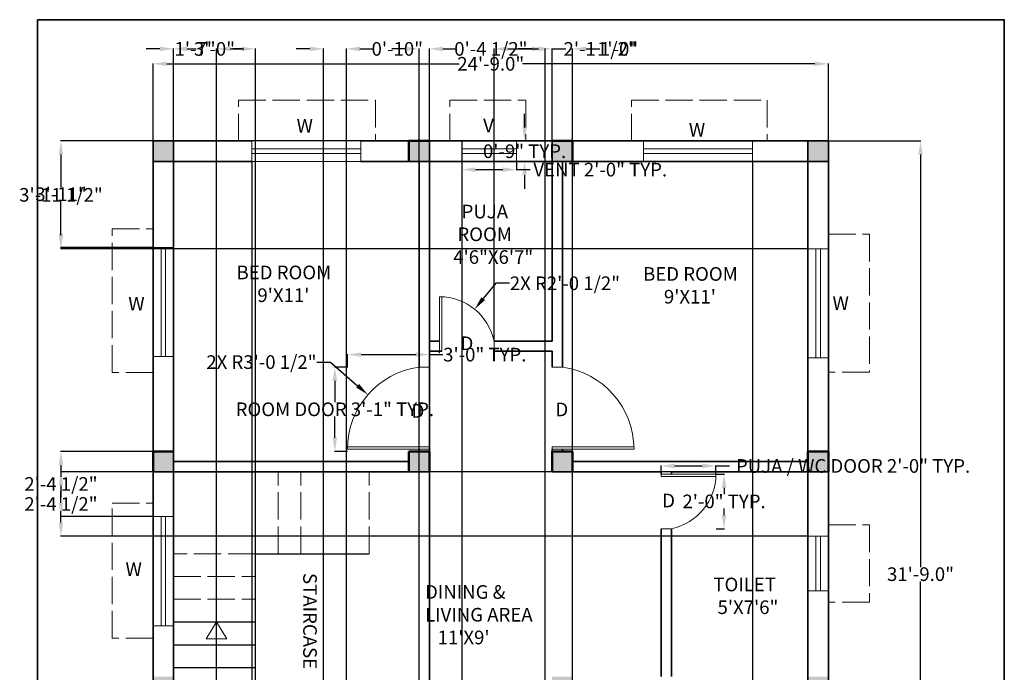
# Model space of a CAD drawing. Units: inches. Extents: x 730 to 1163, y 1530 to 2018.
# Tile 2 of 2: x 730 to 1163, y 1731 to 2018. Entities that reach past the tile are written whole.
import ezdxf

# ---------------------------------------------------------------- set-up
doc = ezdxf.new("R2010")
doc.units = ezdxf.units.IN
doc.header["$MEASUREMENT"] = 0
doc.linetypes.add('ACAD_ISO02W100', pattern=[15, 12, -3])
for name, color, linetype, lineweight in [('A-ANNO-DIMS', 2, 'Continuous', 18), ('A-ANNO-SYMB', 7, 'Continuous', 18), ('A-ANNO-TEXT', 7, 'Continuous', 18), ('A-ANNO-TTLB', 7, 'Continuous', 35), ('A-AREA-IDEN', 7, 'Continuous', 20), ('A-COLS', 7, 'Continuous', 50), ('A-COLS-PATT', 5, 'Continuous', 13), ('A-DOOR', 5, 'Continuous', 18), ('A-FLOR-STRS', 7, 'Continuous', 25), ('A-FLOR-STRS-OVHD', 7, 'ACAD_ISO02W100', 18), ('A-GLAZ', 5, 'Continuous', 18), ('A-GLAZ-OVHD', 7, 'ACAD_ISO02W100', 13), ('A-WALL', 7, 'Continuous', 35)]:
    doc.layers.add(name, color=color, linetype=linetype, lineweight=lineweight)
doc.styles.get("Standard").update_dxf_attribs({"font": 'arial.ttf'})
doc.dimstyles.get("Standard").update_dxf_attribs({"dimtxt": 6, "dimasz": 6, "dimexe": 0.18, "dimexo": 0.0625, "dimgap": 0.09, "dimtad": 0, "dimtih": 1, "dimtoh": 1, "dimdec": 1, "dimzin": 0, "dimdsep": 46, "dimlunit": 3, "dimtxsty": 'Standard', "dimcen": 0.09, "dimclrt": 1, "dimadec": 0, "dimazin": 0, "dimtfac": 1, "dimtdec": 1, "dimtofl": 0, "dimtmove": 0, "dimatfit": 3, "dimfxl": 1, "dimtolj": 1, "dimtzin": 0, "dimarcsym": 0})

# ---------------------------------------------------------------- blocks, each defined once
blk = doc.blocks.new('*D1')
at = {"layer": 'A-ANNO-DIMS', "color": 0, "lineweight": -2, "transparency": 16777216}
for p, q in [((788.44, 1964.64), (788.44, 1998.7)), ((794.44, 1998.52), (923, 1998.52)), ((1079.44, 1998.52), (950.88, 1998.52)), ((1085.44, 1964.64), (1085.44, 1998.7))]:
    blk.add_line(p, q, dxfattribs=at)
at = {"layer": 'A-ANNO-DIMS', "color": 0, "transparency": 16777216}
for points in [[(794.44, 1999.52), (794.44, 1997.52), (788.44, 1998.52)], [(1079.44, 1999.52), (1079.44, 1997.52), (1085.44, 1998.52)]]:
    blk.add_solid(points, dxfattribs=at)
at = {"layer": 'Defpoints', "color": 0, "transparency": 16777216}
for p in [(1085.44, 1998.52), (788.44, 1964.58), (1085.44, 1964.58)]:
    blk.add_point(p, dxfattribs=at)
at = {"layer": 'A-ANNO-DIMS', "color": 0, "transparency": 16777216, "insert": (936.94, 1998.52), "char_height": 6, "attachment_point": 5}
blk.add_mtext('\\A1;24\'-9.0"', dxfattribs=at)
blk = doc.blocks.new('*D2')
at = {"layer": 'A-ANNO-DIMS', "color": 0, "lineweight": -2, "transparency": 16777216}
for p, q in [((1085.5, 1964.58), (1126.1, 1964.58)), ((1125.92, 1958.58), (1125.92, 1777.23)), ((1125.92, 1589.58), (1125.92, 1770.92)), ((1085.5, 1583.58), (1126.1, 1583.58))]:
    blk.add_line(p, q, dxfattribs=at)
at = {"layer": 'A-ANNO-DIMS', "color": 0, "transparency": 16777216}
for points in [[(1124.92, 1958.58), (1126.92, 1958.58), (1125.92, 1964.58)], [(1124.92, 1589.58), (1126.92, 1589.58), (1125.92, 1583.58)]]:
    blk.add_solid(points, dxfattribs=at)
at = {"layer": 'Defpoints', "color": 0, "transparency": 16777216}
for p in [(1085.44, 1964.58), (1085.44, 1583.58), (1125.92, 1583.58)]:
    blk.add_point(p, dxfattribs=at)
at = {"layer": 'A-ANNO-DIMS', "color": 0, "transparency": 16777216, "insert": (1125.92, 1774.08), "char_height": 6, "attachment_point": 5}
blk.add_mtext('\\A1;31\'-9.0"', dxfattribs=at)
blk = doc.blocks.new('WINDOW-48IN')
for p, q in [((0, 9), (0, 0)), ((0, 9), (48, 9)), ((48, 0), (48, 9)), ((0, 5.5), (48, 5.5)), ((0, 3.5), (48, 3.5)), ((0, 0), (48, 0))]:
    blk.add_line(p, q)
blk = doc.blocks.new('VENT-24IN')
for p, q in [((0, 9), (0, 0)), ((24, 9), (0, 9)), ((24, 0), (24, 9)), ((24, 5.5), (0, 5.5)), ((0, 3.5), (24, 3.5)), ((0, 0), (24, 0))]:
    blk.add_line(p, q)
blk = doc.blocks.new('DOOR-SWING-36IN')
for p, q in [((36, 37), (31.5, 37)), ((0, 2), (36, 2)), ((36, 1), (0, 1)), ((0, 1), (36, 1)), ((36, 0), (36, 2))]:
    blk.add_line(p, q)
blk.add_arc((36.32, 1), 36.32, 97.6281, 180)
blk = doc.blocks.new('DOOR-SWING-24IN')
for p, q in [((0, 0), (0, 24)), ((0, 24), (0, 0)), ((1, 24), (1, 0)), ((24, 0), (24, 4.5))]:
    blk.add_line(p, q)
blk.add_arc((0, -0.52), 24.52, 11.8123, 90)
blk = doc.blocks.new('*D9')
at = {"layer": 'A-ANNO-DIMS', "color": 0, "lineweight": -2, "transparency": 16777216}
for p, q in [((924.22, 1955.51), (924.22, 1951.8)), ((948.22, 1955.51), (948.22, 1951.8)), ((930.22, 1951.98), (942.22, 1951.98)), ((948.22, 1951.98), (954.22, 1951.98))]:
    blk.add_line(p, q, dxfattribs=at)
at = {"layer": 'A-ANNO-DIMS', "color": 0, "transparency": 16777216}
for points in [[(930.22, 1952.98), (930.22, 1950.98), (924.22, 1951.98)], [(942.22, 1952.98), (942.22, 1950.98), (948.22, 1951.98)]]:
    blk.add_solid(points, dxfattribs=at)
at = {"layer": 'Defpoints', "color": 0, "transparency": 16777216}
for p in [(924.22, 1955.58), (948.22, 1955.58), (948.22, 1951.98)]:
    blk.add_point(p, dxfattribs=at)
at = {"layer": 'A-ANNO-DIMS', "color": 1, "transparency": 16777216, "insert": (985.09, 1951.98), "char_height": 6, "attachment_point": 5}
blk.add_mtext('\\A1;VENT 2\'-0" TYP.', dxfattribs=at)
blk = doc.blocks.new('*D10')
at = {"layer": 'A-ANNO-DIMS', "color": 0, "lineweight": -2, "transparency": 16777216}
for p, q in [((951.82, 1970.58), (951.82, 1976.58)), ((948.28, 1964.58), (952, 1964.58)), ((948.28, 1955.58), (952, 1955.58)), ((951.82, 1949.58), (951.82, 1943.58))]:
    blk.add_line(p, q, dxfattribs=at)
at = {"layer": 'A-ANNO-DIMS', "color": 0, "transparency": 16777216}
for points in [[(950.82, 1970.58), (952.82, 1970.58), (951.82, 1964.58)], [(950.82, 1949.58), (952.82, 1949.58), (951.82, 1955.58)]]:
    blk.add_solid(points, dxfattribs=at)
at = {"layer": 'Defpoints', "color": 0, "transparency": 16777216}
for p in [(948.22, 1964.58), (951.82, 1964.58), (948.22, 1955.58)]:
    blk.add_point(p, dxfattribs=at)
at = {"layer": 'A-ANNO-DIMS', "color": 1, "transparency": 16777216, "insert": (951.82, 1960.08), "char_height": 6, "attachment_point": 5}
blk.add_mtext('\\A1;0\'-9" TYP.', dxfattribs=at)
blk = doc.blocks.new('*D11')
at = {"layer": 'A-ANNO-DIMS', "color": 0, "lineweight": -2, "transparency": 16777216}
for p, q in [((873.88, 1865.08), (868.21, 1865.08)), ((868.39, 1859.08), (868.39, 1849.77)), ((868.39, 1834.08), (868.39, 1843.38)), ((873.88, 1828.08), (868.21, 1828.08))]:
    blk.add_line(p, q, dxfattribs=at)
at = {"layer": 'A-ANNO-DIMS', "color": 0, "transparency": 16777216}
for points in [[(867.39, 1859.08), (869.39, 1859.08), (868.39, 1865.08)], [(867.39, 1834.08), (869.39, 1834.08), (868.39, 1828.08)]]:
    blk.add_solid(points, dxfattribs=at)
at = {"layer": 'Defpoints', "color": 0, "transparency": 16777216}
for p in [(868.39, 1865.08), (873.94, 1865.08), (873.94, 1828.08)]:
    blk.add_point(p, dxfattribs=at)
at = {"layer": 'A-ANNO-DIMS', "color": 1, "transparency": 16777216, "insert": (868.39, 1846.58), "char_height": 6, "attachment_point": 5}
blk.add_mtext('\\A1;ROOM DOOR 3\'-1" TYP.', dxfattribs=at)
blk = doc.blocks.new('*D12')
at = {"layer": 'A-ANNO-DIMS', "color": 0, "lineweight": -2, "transparency": 16777216}
for p, q in [((873.94, 1865.14), (873.94, 1870.81)), ((879.94, 1870.63), (903.94, 1870.63)), ((909.94, 1865.14), (909.94, 1870.81)), ((909.94, 1870.63), (915.94, 1870.63))]:
    blk.add_line(p, q, dxfattribs=at)
at = {"layer": 'A-ANNO-DIMS', "color": 0, "transparency": 16777216}
for points in [[(879.94, 1871.63), (879.94, 1869.63), (873.94, 1870.63)], [(903.94, 1871.63), (903.94, 1869.63), (909.94, 1870.63)]]:
    blk.add_solid(points, dxfattribs=at)
at = {"layer": 'Defpoints', "color": 0, "transparency": 16777216}
for p in [(909.94, 1870.63), (873.94, 1865.08), (909.94, 1865.08)]:
    blk.add_point(p, dxfattribs=at)
at = {"layer": 'A-ANNO-DIMS', "color": 1, "transparency": 16777216, "insert": (934.32, 1870.63), "char_height": 6, "attachment_point": 5}
blk.add_mtext('\\A1;3\'-0" TYP.', dxfattribs=at)
blk = doc.blocks.new('*D13')
at = {"layer": 'A-ANNO-DIMS', "color": 0, "lineweight": -2, "transparency": 16777216}
for p, q in [((1011.94, 1818.14), (1011.94, 1821.86)), ((1017.94, 1821.68), (1029.94, 1821.68)), ((1035.94, 1818.14), (1035.94, 1821.86)), ((1035.94, 1821.68), (1041.94, 1821.68))]:
    blk.add_line(p, q, dxfattribs=at)
at = {"layer": 'A-ANNO-DIMS', "color": 0, "transparency": 16777216}
for points in [[(1017.94, 1822.68), (1017.94, 1820.68), (1011.94, 1821.68)], [(1029.94, 1822.68), (1029.94, 1820.68), (1035.94, 1821.68)]]:
    blk.add_solid(points, dxfattribs=at)
at = {"layer": 'Defpoints', "color": 0, "transparency": 16777216}
for p in [(1035.94, 1821.68), (1011.94, 1818.08), (1035.94, 1818.08)]:
    blk.add_point(p, dxfattribs=at)
at = {"layer": 'A-ANNO-DIMS', "color": 1, "transparency": 16777216, "insert": (1096.26, 1821.68), "char_height": 6, "attachment_point": 5}
blk.add_mtext('\\A1;PUJA / WC DOOR 2\'-0" TYP.', dxfattribs=at)
blk = doc.blocks.new('*D14')
at = {"layer": 'A-ANNO-DIMS', "color": 0, "lineweight": -2, "transparency": 16777216}
for p, q in [((1036, 1818.08), (1039.72, 1818.08)), ((1039.54, 1812.08), (1039.54, 1809.23)), ((1039.54, 1800.08), (1039.54, 1802.92)), ((1036, 1794.08), (1039.72, 1794.08))]:
    blk.add_line(p, q, dxfattribs=at)
at = {"layer": 'A-ANNO-DIMS', "color": 0, "transparency": 16777216}
for points in [[(1038.54, 1812.08), (1040.54, 1812.08), (1039.54, 1818.08)], [(1038.54, 1800.08), (1040.54, 1800.08), (1039.54, 1794.08)]]:
    blk.add_solid(points, dxfattribs=at)
at = {"layer": 'Defpoints', "color": 0, "transparency": 16777216}
for p in [(1035.94, 1818.08), (1035.94, 1794.08), (1039.54, 1794.08)]:
    blk.add_point(p, dxfattribs=at)
at = {"layer": 'A-ANNO-DIMS', "color": 1, "transparency": 16777216, "insert": (1039.54, 1806.08), "char_height": 6, "attachment_point": 5}
blk.add_mtext('\\A1;2\'-0" TYP.', dxfattribs=at)
blk = doc.blocks.new('*D15')
at = {"layer": 'A-ANNO-DIMS', "color": 0, "lineweight": -2, "transparency": 16777216}
for p, q in [((797.44, 1964.51), (797.44, 1540.9)), ((831.86, 1955.51), (831.86, 1540.9)), ((803.44, 1541.08), (825.86, 1541.08)), ((831.86, 1541.08), (837.86, 1541.08))]:
    blk.add_line(p, q, dxfattribs=at)
at = {"layer": 'A-ANNO-DIMS', "color": 0, "transparency": 16777216}
for points in [[(803.44, 1542.08), (803.44, 1540.08), (797.44, 1541.08)], [(825.86, 1542.08), (825.86, 1540.08), (831.86, 1541.08)]]:
    blk.add_solid(points, dxfattribs=at)
at = {"layer": 'Defpoints', "color": 0, "transparency": 16777216}
for p in [(797.44, 1964.58), (831.86, 1955.58), (831.86, 1541.08)]:
    blk.add_point(p, dxfattribs=at)
at = {"layer": 'A-ANNO-DIMS', "color": 1, "transparency": 16777216, "insert": (855.3, 1541.08), "char_height": 6, "attachment_point": 5}
blk.add_mtext('\\A1;2\'-10 1/2"', dxfattribs=at)
blk = doc.blocks.new('*D16')
at = {"layer": 'A-ANNO-DIMS', "color": 0, "lineweight": -2, "transparency": 16777216}
for p, q in [((909.94, 1964.51), (909.94, 1540.9)), ((924.22, 1964.51), (924.22, 1540.9)), ((915.94, 1541.08), (918.22, 1541.08)), ((924.22, 1541.08), (930.22, 1541.08))]:
    blk.add_line(p, q, dxfattribs=at)
at = {"layer": 'A-ANNO-DIMS', "color": 0, "transparency": 16777216}
for points in [[(915.94, 1542.08), (915.94, 1540.08), (909.94, 1541.08)], [(918.22, 1542.08), (918.22, 1540.08), (924.22, 1541.08)]]:
    blk.add_solid(points, dxfattribs=at)
at = {"layer": 'Defpoints', "color": 0, "transparency": 16777216}
for p in [(909.94, 1964.58), (924.22, 1964.58), (924.22, 1541.08)]:
    blk.add_point(p, dxfattribs=at)
at = {"layer": 'A-ANNO-DIMS', "color": 1, "transparency": 16777216, "insert": (944.99, 1541.08), "char_height": 6, "attachment_point": 5}
blk.add_mtext('\\A1;1\'-2 1/2"', dxfattribs=at)
blk = doc.blocks.new('*D17')
at = {"layer": 'A-ANNO-DIMS', "color": 0, "lineweight": -2, "transparency": 16777216}
for p, q in [((1076.44, 1964.51), (1076.44, 1540.9)), ((1052.04, 1955.51), (1052.04, 1540.9)), ((1058.04, 1541.08), (1070.44, 1541.08)), ((1076.44, 1541.08), (1082.44, 1541.08))]:
    blk.add_line(p, q, dxfattribs=at)
at = {"layer": 'A-ANNO-DIMS', "color": 0, "transparency": 16777216}
for points in [[(1058.04, 1542.08), (1058.04, 1540.08), (1052.04, 1541.08)], [(1070.44, 1542.08), (1070.44, 1540.08), (1076.44, 1541.08)]]:
    blk.add_solid(points, dxfattribs=at)
at = {"layer": 'Defpoints', "color": 0, "transparency": 16777216}
for p in [(1076.44, 1964.58), (1052.04, 1955.58), (1076.44, 1541.08)]:
    blk.add_point(p, dxfattribs=at)
at = {"layer": 'A-ANNO-DIMS', "color": 1, "transparency": 16777216, "insert": (1097.55, 1541.08), "char_height": 6, "attachment_point": 5}
blk.add_mtext('\\A1;2\'-0 1/2"', dxfattribs=at)
blk = doc.blocks.new('*D18')
at = {"layer": 'A-ANNO-DIMS', "color": 0, "lineweight": -2, "transparency": 16777216}
for p, q in [((788.38, 1964.58), (747.76, 1964.58)), ((747.94, 1958.58), (747.94, 1944.35)), ((747.94, 1923.81), (747.94, 1938.04)), ((788.38, 1917.81), (747.76, 1917.81))]:
    blk.add_line(p, q, dxfattribs=at)
at = {"layer": 'A-ANNO-DIMS', "color": 0, "transparency": 16777216}
for points in [[(746.94, 1958.58), (748.94, 1958.58), (747.94, 1964.58)], [(746.94, 1923.81), (748.94, 1923.81), (747.94, 1917.81)]]:
    blk.add_solid(points, dxfattribs=at)
at = {"layer": 'Defpoints', "color": 0, "transparency": 16777216}
for p in [(788.44, 1964.58), (747.94, 1917.81), (788.44, 1917.81)]:
    blk.add_point(p, dxfattribs=at)
at = {"layer": 'A-ANNO-DIMS', "color": 1, "transparency": 16777216, "insert": (747.94, 1941.19), "char_height": 6, "attachment_point": 5}
blk.add_mtext('\\A1;3\'-11"', dxfattribs=at)
blk = doc.blocks.new('*D19')
at = {"layer": 'A-ANNO-DIMS', "color": 0, "lineweight": -2, "transparency": 16777216}
for p, q in [((788.38, 1828.08), (747.76, 1828.08)), ((747.94, 1822.08), (747.94, 1816.93)), ((747.94, 1805.4), (747.94, 1810.54)), ((788.38, 1799.4), (747.76, 1799.4))]:
    blk.add_line(p, q, dxfattribs=at)
at = {"layer": 'A-ANNO-DIMS', "color": 0, "transparency": 16777216}
for points in [[(746.94, 1822.08), (748.94, 1822.08), (747.94, 1828.08)], [(746.94, 1805.4), (748.94, 1805.4), (747.94, 1799.4)]]:
    blk.add_solid(points, dxfattribs=at)
at = {"layer": 'Defpoints', "color": 0, "transparency": 16777216}
for p in [(788.44, 1828.08), (747.94, 1799.4), (788.44, 1799.4)]:
    blk.add_point(p, dxfattribs=at)
at = {"layer": 'A-ANNO-DIMS', "color": 1, "transparency": 16777216, "insert": (747.94, 1813.74), "char_height": 6, "attachment_point": 5}
blk.add_mtext('\\A1;2\'-4 1/2"', dxfattribs=at)
blk = doc.blocks.new('*D21')
at = {"layer": 'A-ANNO-DIMS', "color": 0, "lineweight": -2, "transparency": 16777216}
for p, q in [((1076.38, 1964.58), (747.76, 1964.58)), ((747.94, 1958.58), (747.94, 1944.08)), ((747.94, 1923.2), (747.94, 1937.69)), ((1076.38, 1917.2), (747.76, 1917.2))]:
    blk.add_line(p, q, dxfattribs=at)
at = {"layer": 'A-ANNO-DIMS', "color": 0, "transparency": 16777216}
for points in [[(746.94, 1958.58), (748.94, 1958.58), (747.94, 1964.58)], [(746.94, 1923.2), (748.94, 1923.2), (747.94, 1917.2)]]:
    blk.add_solid(points, dxfattribs=at)
at = {"layer": 'Defpoints', "color": 0, "transparency": 16777216}
for p in [(1076.44, 1964.58), (747.94, 1917.2), (1076.44, 1917.2)]:
    blk.add_point(p, dxfattribs=at)
at = {"layer": 'A-ANNO-DIMS', "color": 1, "transparency": 16777216, "insert": (747.94, 1940.89), "char_height": 6, "attachment_point": 5}
blk.add_mtext('\\A1;3\'-11 1/2"', dxfattribs=at)
blk = doc.blocks.new('*D22')
at = {"layer": 'A-ANNO-DIMS', "color": 0, "lineweight": -2, "transparency": 16777216}
for p, q in [((1076.38, 1819.08), (747.76, 1819.08)), ((747.94, 1813.08), (747.94, 1808.13)), ((747.94, 1796.8), (747.94, 1801.75)), ((1076.38, 1790.8), (747.76, 1790.8))]:
    blk.add_line(p, q, dxfattribs=at)
at = {"layer": 'A-ANNO-DIMS', "color": 0, "transparency": 16777216}
for points in [[(746.94, 1813.08), (748.94, 1813.08), (747.94, 1819.08)], [(746.94, 1796.8), (748.94, 1796.8), (747.94, 1790.8)]]:
    blk.add_solid(points, dxfattribs=at)
at = {"layer": 'Defpoints', "color": 0, "transparency": 16777216}
for p in [(747.94, 1819.08), (1076.44, 1819.08), (1076.44, 1790.8)]:
    blk.add_point(p, dxfattribs=at)
at = {"layer": 'A-ANNO-DIMS', "color": 1, "transparency": 16777216, "insert": (747.94, 1804.94), "char_height": 6, "attachment_point": 5}
blk.add_mtext('\\A1;2\'-4 1/2"', dxfattribs=at)
blk = doc.blocks.new('*D27')
at = {"layer": 'A-ANNO-DIMS', "color": 0, "lineweight": -2, "transparency": 16777216}
for p, q in [((797.44, 1733.14), (797.44, 2005.26)), ((803.44, 2005.08), (807.38, 2005.08)), ((827.44, 2005.08), (823.5, 2005.08)), ((833.44, 1733.14), (833.44, 2005.26))]:
    blk.add_line(p, q, dxfattribs=at)
at = {"layer": 'A-ANNO-DIMS', "color": 0, "transparency": 16777216}
for points in [[(803.44, 2006.08), (803.44, 2004.08), (797.44, 2005.08)], [(827.44, 2006.08), (827.44, 2004.08), (833.44, 2005.08)]]:
    blk.add_solid(points, dxfattribs=at)
at = {"layer": 'Defpoints', "color": 0, "transparency": 16777216}
for p in [(833.44, 2005.08), (797.44, 1733.08), (833.44, 1733.08)]:
    blk.add_point(p, dxfattribs=at)
at = {"layer": 'A-ANNO-DIMS', "color": 1, "transparency": 16777216, "insert": (815.44, 2005.08), "char_height": 6, "attachment_point": 5}
blk.add_mtext('\\A1;3\'-0"', dxfattribs=at)
blk = doc.blocks.new('*D28')
at = {"layer": 'A-ANNO-DIMS', "color": 0, "lineweight": -2, "transparency": 16777216}
for p, q in [((857.44, 2005.08), (851.44, 2005.08)), ((863.44, 1721.06), (863.44, 2005.26)), ((873.44, 1721.06), (873.44, 2005.26)), ((879.44, 2005.08), (885.44, 2005.08))]:
    blk.add_line(p, q, dxfattribs=at)
at = {"layer": 'A-ANNO-DIMS', "color": 0, "transparency": 16777216}
for points in [[(857.44, 2006.08), (857.44, 2004.08), (863.44, 2005.08)], [(879.44, 2006.08), (879.44, 2004.08), (873.44, 2005.08)]]:
    blk.add_solid(points, dxfattribs=at)
at = {"layer": 'Defpoints', "color": 0, "transparency": 16777216}
for p in [(873.44, 2005.08), (863.44, 1721), (873.44, 1721)]:
    blk.add_point(p, dxfattribs=at)
at = {"layer": 'A-ANNO-DIMS', "color": 1, "transparency": 16777216, "insert": (895.84, 2005.08), "char_height": 6, "attachment_point": 5}
blk.add_mtext('\\A1;0\'-10"', dxfattribs=at)
blk = doc.blocks.new('*D32')
at = {"layer": 'A-ANNO-DIMS', "color": 0, "lineweight": -2, "transparency": 16777216}
for p, q in [((791.44, 2005.08), (785.44, 2005.08)), ((797.44, 1605.26), (797.44, 2005.26)), ((816.4, 1613.85), (816.4, 2005.26)), ((822.4, 2005.08), (828.4, 2005.08))]:
    blk.add_line(p, q, dxfattribs=at)
at = {"layer": 'A-ANNO-DIMS', "color": 0, "transparency": 16777216}
for points in [[(791.44, 2006.08), (791.44, 2004.08), (797.44, 2005.08)], [(822.4, 2006.08), (822.4, 2004.08), (816.4, 2005.08)]]:
    blk.add_solid(points, dxfattribs=at)
at = {"layer": 'Defpoints', "color": 0, "transparency": 16777216}
for p in [(816.4, 2005.08), (816.4, 1613.79), (797.44, 1605.2)]:
    blk.add_point(p, dxfattribs=at)
at = {"layer": 'A-ANNO-DIMS', "color": 1, "transparency": 16777216, "insert": (806.92, 2005.08), "char_height": 6, "attachment_point": 5}
blk.add_mtext('\\A1;1\'-7"', dxfattribs=at)
blk = doc.blocks.new('*D34')
at = {"layer": 'A-ANNO-DIMS', "color": 0, "lineweight": -2, "transparency": 16777216}
for p, q in [((899.44, 2005.08), (893.44, 2005.08)), ((905.44, 1592.64), (905.44, 2005.26)), ((909.94, 1592.64), (909.94, 2005.26)), ((915.94, 2005.08), (921.94, 2005.08))]:
    blk.add_line(p, q, dxfattribs=at)
at = {"layer": 'A-ANNO-DIMS', "color": 0, "transparency": 16777216}
for points in [[(899.44, 2006.08), (899.44, 2004.08), (905.44, 2005.08)], [(915.94, 2006.08), (915.94, 2004.08), (909.94, 2005.08)]]:
    blk.add_solid(points, dxfattribs=at)
at = {"layer": 'Defpoints', "color": 0, "transparency": 16777216}
for p in [(909.94, 2005.08), (905.44, 1592.58), (909.94, 1592.58)]:
    blk.add_point(p, dxfattribs=at)
at = {"layer": 'A-ANNO-DIMS', "color": 1, "transparency": 16777216, "insert": (937, 2005.08), "char_height": 6, "attachment_point": 5}
blk.add_mtext('\\A1;0\'-4 1/2"', dxfattribs=at)
blk = doc.blocks.new('*D36')
at = {"layer": 'A-ANNO-DIMS', "color": 0, "lineweight": -2, "transparency": 16777216}
for p, q in [((954.94, 2005.08), (948.94, 2005.08)), ((960.94, 1583.64), (960.94, 2005.26)), ((972.94, 1583.64), (972.94, 2005.26)), ((978.94, 2005.08), (984.94, 2005.08))]:
    blk.add_line(p, q, dxfattribs=at)
at = {"layer": 'A-ANNO-DIMS', "color": 0, "transparency": 16777216}
for points in [[(954.94, 2006.08), (954.94, 2004.08), (960.94, 2005.08)], [(978.94, 2006.08), (978.94, 2004.08), (972.94, 2005.08)]]:
    blk.add_solid(points, dxfattribs=at)
at = {"layer": 'Defpoints', "color": 0, "transparency": 16777216}
for p in [(972.94, 2005.08), (960.94, 1583.58), (972.94, 1583.58)]:
    blk.add_point(p, dxfattribs=at)
at = {"layer": 'A-ANNO-DIMS', "color": 1, "transparency": 16777216, "insert": (992.72, 2005.08), "char_height": 6, "attachment_point": 5}
blk.add_mtext('\\A1;1\'-0"', dxfattribs=at)
blk = doc.blocks.new('*D37')
at = {"layer": 'A-ANNO-DIMS', "color": 0, "lineweight": -2, "transparency": 16777216}
for p, q in [((938.38, 1876.64), (938.38, 2005.26)), ((944.38, 2005.08), (957.94, 2005.08)), ((963.94, 1876.64), (963.94, 2005.26)), ((963.94, 2005.08), (969.94, 2005.08))]:
    blk.add_line(p, q, dxfattribs=at)
at = {"layer": 'A-ANNO-DIMS', "color": 0, "transparency": 16777216}
for points in [[(944.38, 2006.08), (944.38, 2004.08), (938.38, 2005.08)], [(957.94, 2006.08), (957.94, 2004.08), (963.94, 2005.08)]]:
    blk.add_solid(points, dxfattribs=at)
at = {"layer": 'Defpoints', "color": 0, "transparency": 16777216}
for p in [(963.94, 2005.08), (938.38, 1876.58), (963.94, 1876.58)]:
    blk.add_point(p, dxfattribs=at)
at = {"layer": 'A-ANNO-DIMS', "color": 1, "transparency": 16777216, "insert": (985.05, 2005.08), "char_height": 6, "attachment_point": 5}
blk.add_mtext('\\A1;2\'-1 1/2"', dxfattribs=at)
blk = doc.blocks.new('*D38')
at = {"layer": 'A-ANNO-DIMS', "color": 0, "lineweight": -2, "transparency": 16777216}
for p, q in [((860.53, 1867.35), (866.53, 1867.35)), ((866.53, 1867.35), (878.41, 1856.95)), ((910.17, 1829.08), (910.35, 1829.08)), ((910.26, 1828.99), (910.26, 1829.17))]:
    blk.add_line(p, q, dxfattribs=at)
at = {"layer": 'A-ANNO-DIMS', "color": 0, "transparency": 16777216}
blk.add_solid([(879.07, 1857.7), (877.76, 1856.19), (882.93, 1852.99)], dxfattribs=at)
at = {"layer": 'Defpoints', "color": 0, "transparency": 16777216}
for p in [(882.93, 1852.99), (910.26, 1829.08)]:
    blk.add_point(p, dxfattribs=at)
at = {"layer": 'A-ANNO-DIMS', "color": 1, "transparency": 16777216, "insert": (836.1, 1867.35), "char_height": 6, "attachment_point": 5}
blk.add_mtext('\\A1;2X R3\'-0 1/2"', dxfattribs=at)
blk = doc.blocks.new('*D40')
at = {"layer": 'A-ANNO-DIMS', "color": 0, "lineweight": -2, "transparency": 16777216}
for p, q in [((939.12, 1902.01), (933.63, 1895.24)), ((945.12, 1902.01), (939.12, 1902.01)), ((914.29, 1871.56), (914.47, 1871.56)), ((914.38, 1871.47), (914.38, 1871.65))]:
    blk.add_line(p, q, dxfattribs=at)
at = {"layer": 'A-ANNO-DIMS', "color": 0, "transparency": 16777216}
blk.add_solid([(932.85, 1895.87), (934.41, 1894.61), (929.85, 1890.59)], dxfattribs=at)
at = {"layer": 'Defpoints', "color": 0, "transparency": 16777216}
for p in [(929.85, 1890.59), (914.38, 1871.56)]:
    blk.add_point(p, dxfattribs=at)
at = {"layer": 'A-ANNO-DIMS', "color": 1, "transparency": 16777216, "insert": (969.55, 1902.01), "char_height": 6, "attachment_point": 5}
blk.add_mtext('\\A1;2X R2\'-0 1/2"', dxfattribs=at)

msp = doc.modelspace()

# ---------------------------------------------------------------- hatches: boundary and pattern name
at = {"layer": 'A-COLS-PATT'}
h = msp.add_hatch(color=256, dxfattribs=at)
h.dxf.hatch_style = 1
h.paths.add_polyline_path([(797.44, 1964.58), (788.44, 1964.58), (788.44, 1955.58), (797.44, 1955.58)])
h.paths.add_polyline_path([(909.94, 1964.58), (900.94, 1964.58), (900.94, 1955.58), (909.94, 1955.58)])
h.paths.add_polyline_path([(972.94, 1964.58), (963.94, 1964.58), (963.94, 1955.58), (972.94, 1955.58)])
h.paths.add_polyline_path([(1085.44, 1964.58), (1076.44, 1964.58), (1076.44, 1955.58), (1085.44, 1955.58)])
h.paths.add_polyline_path([(797.44, 1828.08), (788.44, 1828.08), (788.44, 1819.08), (797.44, 1819.08)])
h.paths.add_polyline_path([(909.94, 1828.08), (900.94, 1828.08), (900.94, 1819.08), (909.94, 1819.08)])
h.paths.add_polyline_path([(972.94, 1828.08), (963.94, 1828.08), (963.94, 1819.08), (972.94, 1819.08)])
h.paths.add_polyline_path([(1085.44, 1828.08), (1076.44, 1828.08), (1076.44, 1819.08), (1085.44, 1819.08)])
h.paths.add_polyline_path([(797.44, 1729.08), (788.44, 1729.08), (788.44, 1720.08), (797.44, 1720.08)])
h.paths.add_polyline_path([(972.96, 1729.08), (963.94, 1729.08), (963.94, 1720.07), (972.96, 1720.07)])
h.paths.add_polyline_path([(1085.44, 1729.08), (1076.44, 1729.08), (1076.44, 1720.08), (1085.44, 1720.08)])
h.paths.add_polyline_path([(1085.44, 1592.58), (1076.44, 1592.58), (1076.44, 1583.58), (1085.44, 1583.58)])
h.paths.add_polyline_path([(972.94, 1592.58), (963.94, 1592.58), (963.94, 1583.58), (972.94, 1583.58)])
h.paths.add_polyline_path([(909.94, 1592.58), (900.94, 1592.58), (900.94, 1583.58), (909.94, 1583.58)])
h.paths.add_polyline_path([(797.44, 1592.58), (788.44, 1592.58), (788.44, 1583.58), (797.44, 1583.58)])

# ---------------------------------------------------------------- linework, layer by layer
at = {"layer": 'A-ANNO-SYMB'}
for p, q in [((816.36, 1753.08), (811.77, 1745.67)), ((816.36, 1753.08), (820.95, 1745.67)), ((811.77, 1745.67), (820.95, 1745.67)), ((816.36, 1701.04), (816.36, 1745.67))]:
    msp.add_line(p, q, dxfattribs=at)
at = {"layer": 'A-ANNO-TTLB'}
msp.add_lwpolyline([(737.62, 2017.92), (1162.77, 2017.92), (1162.77, 1530.25), (737.62, 1530.25)], close=True, dxfattribs=at)
at = {"layer": 'A-COLS'}
for p, q in [((909.94, 1964.58), (900.94, 1964.58)), ((900.94, 1964.58), (900.94, 1955.58)), ((963.94, 1964.58), (972.94, 1964.58)), ((972.94, 1964.58), (972.94, 1955.58)), ((788.44, 1819.08), (788.44, 1828.08)), ((788.44, 1828.08), (797.44, 1828.08)), ((909.94, 1828.08), (900.94, 1828.08)), ((900.94, 1828.08), (900.94, 1819.08)), ((909.94, 1819.08), (909.94, 1828.08)), ((963.94, 1819.08), (963.94, 1828.08)), ((963.94, 1828.08), (972.94, 1828.08)), ((972.94, 1828.08), (972.94, 1819.08)), ((1085.44, 1828.08), (1076.44, 1828.08)), ((1076.44, 1828.08), (1076.44, 1819.08)), ((1085.44, 1819.08), (1085.44, 1828.08))]:
    msp.add_line(p, q, dxfattribs=at)
at = {"layer": 'A-DOOR'}
msp.add_line((1011.94, 1819.08), (1011.94, 1817.08), dxfattribs=at)
at = {"layer": 'A-FLOR-STRS'}
for p, q in [((797.44, 1819.08), (797.44, 1783.08)), ((833.44, 1783.08), (883.44, 1783.08)), ((833.44, 1681.08), (833.44, 1783.08)), ((797.44, 1753.08), (833.44, 1753.08)), ((797.44, 1743.08), (833.44, 1743.08)), ((797.44, 1733.08), (833.44, 1733.08))]:
    msp.add_line(p, q, dxfattribs=at)
at = {"layer": 'A-FLOR-STRS-OVHD'}
for p, q in [((833.44, 1783.08), (833.44, 1819.08)), ((843.44, 1783.08), (843.44, 1819.08)), ((853.44, 1783.08), (853.44, 1819.08)), ((863.44, 1783.08), (863.44, 1819.08)), ((873.44, 1783.08), (873.44, 1819.08)), ((883.44, 1783.08), (883.44, 1819.08)), ((833.44, 1783.08), (797.44, 1783.08)), ((797.44, 1773.08), (833.44, 1773.08)), ((797.44, 1763.08), (833.44, 1763.08))]:
    msp.add_line(p, q, dxfattribs=at)
at = {"layer": 'A-GLAZ-OVHD'}
for p, q in [((826.03, 1964.58), (826.03, 1982.58)), ((826.03, 1982.58), (886.23, 1982.58)), ((886.23, 1982.58), (886.23, 1964.58)), ((918.9, 1964.58), (918.9, 1982.58)), ((918.9, 1982.58), (952.44, 1982.58)), ((952.44, 1982.58), (952.44, 1964.58)), ((998.8, 1964.58), (998.8, 1982.58)), ((998.8, 1982.58), (1058.55, 1982.58)), ((1058.55, 1982.58), (1058.55, 1964.58)), ((770.44, 1862.84), (770.44, 1925.89)), ((770.44, 1925.89), (788.44, 1925.89)), ((1085.44, 1923.62), (1103.44, 1923.62)), ((1103.44, 1923.62), (1103.44, 1862.96)), ((788.44, 1862.84), (770.44, 1862.84)), ((1103.44, 1862.96), (1085.44, 1862.96)), ((770.44, 1745.93), (770.44, 1805.25)), ((770.44, 1805.25), (788.44, 1805.25)), ((1085.44, 1795.74), (1103.44, 1795.74)), ((1103.44, 1795.74), (1103.44, 1761.8)), ((1103.44, 1761.8), (1085.44, 1761.8)), ((788.44, 1745.93), (770.44, 1745.93))]:
    msp.add_line(p, q, dxfattribs=at)
at = {"layer": 'A-WALL'}
for p, q in [((788.44, 1964.58), (831.86, 1964.58)), ((788.44, 1964.58), (788.44, 1583.58)), ((797.44, 1964.58), (797.44, 1681.08)), ((879.86, 1964.58), (1085.44, 1964.58)), ((909.94, 1964.58), (909.94, 1876.58)), ((963.94, 1964.58), (963.94, 1876.58)), ((1076.44, 1964.58), (1076.44, 1583.58)), ((1085.44, 1964.58), (1085.44, 1583.58)), ((788.44, 1955.58), (831.86, 1955.58)), ((879.86, 1955.58), (1085.44, 1955.58)), ((905.44, 1955.58), (905.44, 1865.08)), ((968.44, 1955.58), (968.44, 1865.08)), ((909.94, 1876.58), (914.38, 1876.58)), ((938.38, 1876.58), (963.94, 1876.58)), ((909.94, 1872.08), (915.38, 1872.08)), ((909.94, 1872.08), (909.94, 1865.08)), ((938.38, 1872.08), (963.94, 1872.08)), ((963.94, 1872.08), (963.94, 1865.08)), ((905.44, 1829.08), (905.44, 1828.08)), ((909.94, 1829.08), (909.94, 1819.08)), ((963.94, 1829.08), (963.94, 1819.08)), ((968.44, 1829.08), (968.44, 1828.08)), ((797.44, 1823.58), (900.94, 1823.58)), ((972.94, 1823.58), (1076.44, 1823.58)), ((788.44, 1819.08), (909.94, 1819.08)), ((963.94, 1819.08), (1011.94, 1819.08)), ((1011.94, 1819.08), (1011.94, 1818.08)), ((1016.44, 1819.08), (1016.44, 1818.08)), ((1016.44, 1819.08), (1085.44, 1819.08)), ((1011.94, 1794.08), (1011.94, 1729.08)), ((1016.44, 1794.08), (1016.44, 1729.08))]:
    msp.add_line(p, q, dxfattribs=at)

# ---------------------------------------------------------------- block references
at = {"layer": 'A-DOOR'}
for name, p in [('DOOR-SWING-24IN', (914.38, 1872.08)), ('DOOR-SWING-36IN', (873.94, 1828.08))]:
    msp.add_blockref(name, p, dxfattribs=at)
at = {"layer": 'A-DOOR', "extrusion": (0, 0, -1), "zscale": -1}
msp.add_blockref('DOOR-SWING-36IN', (-999.94, 1828.08), dxfattribs=at)
at = {"layer": 'A-DOOR', "rotation": 270.0000000000006}
msp.add_blockref('DOOR-SWING-24IN', (1011.94, 1818.08), dxfattribs=at)
at = {"layer": 'A-GLAZ'}
for name, p in [('WINDOW-48IN', (831.86, 1955.58)), ('VENT-24IN', (924.22, 1955.58))]:
    msp.add_blockref(name, p, dxfattribs=at)
for name, p, rotation in [('WINDOW-48IN', (1052.04, 1964.58), 180), ('WINDOW-48IN', (797.44, 1869.81), 89.999999999999), ('WINDOW-48IN', (1085.44, 1869.2), 89.9999999999992), ('WINDOW-48IN', (797.44, 1751.4), 89.999999999999), ('VENT-24IN', (1076.44, 1790.8), 270.0000000000011)]:
    msp.add_blockref(name, p, dxfattribs=dict(at, rotation=rotation))

# ---------------------------------------------------------------- texts
at = {"layer": 'A-ANNO-TEXT', "char_height": 6, "attachment_point": 1}
for s, width, insert in [('V', 9.5548, (933.61, 1974.37)), ('W', 10.9415, (851.57, 1974.3)), ('W', 10.9415, (1024.05, 1972.54)), ('W', 10.9415, (777.55, 1896.04)), ('W', 10.9415, (1087.23, 1896.29)), ('D', 6.6774, (923.66, 1878.6)), ('D', 6.6774, (902.12, 1848.9)), ('D', 6.6774, (965.39, 1849.52)), ('D', 6.6774, (1012.34, 1809.46)), ('W', 10.9415, (776.33, 1779.27))]:
    msp.add_mtext_dynamic_manual_height_columns(s, width=width, gutter_width=30, heights=[0], dxfattribs=dict(at, insert=insert))
at = {"layer": 'A-AREA-IDEN', "char_height": 6, "attachment_point": 1}
for s, width, insert in [('  PUJA\\P ROOM\\P4\'6"X6\'7"', 40.4883, (920.44, 1936.55)), ("BED ROOM\\P     9'X11'", 66.8854, (825.16, 1909.76)), ("BED ROOM\\P     9'X11'", 66.8854, (1003.92, 1909.11)), ('TOILET\\P 5\'X7\'6"', 39.6158, (1034.83, 1772.55)), ("DINING &\\PLIVING AREA\\P   11'X9'", 55.789, (908.05, 1769.25))]:
    msp.add_mtext_dynamic_manual_height_columns(s, width=width, gutter_width=30, heights=[0], dxfattribs=dict(at, insert=insert))
at = {"layer": 'A-AREA-IDEN', "insert": (860.46, 1774.58), "char_height": 6, "attachment_point": 1, "rotation": 270}
msp.add_mtext_dynamic_manual_height_columns('STAIRCASE', width=39.9272, gutter_width=30, heights=[0], dxfattribs=at)

# ---------------------------------------------------------------- dimensions: what is measured, and where the dimension line sits
at = {"layer": 'A-ANNO-DIMS'}
for base, p1, p2, override, picture, middle in [((909.94, 2005.08), (905.44, 1592.58), (909.94, 1592.58), {"dimdec": 1, "dimlfac": 1, "dimrnd": 0, "dimzin": 1, "dimdsep": 46, "dimlunit": 4, "dimfrac": 2}, '*D34', (937, 2005.08)), ((963.94, 2005.08), (938.38, 1876.58), (963.94, 1876.58), {"dimdec": 1, "dimlfac": 1, "dimrnd": 0, "dimzin": 1, "dimdsep": 46, "dimlunit": 4, "dimfrac": 2}, '*D37', (985.05, 2005.08)), ((816.4, 2005.08), (797.44, 1605.2), (816.4, 1613.79), {"dimdec": 1, "dimlfac": 1, "dimrnd": 0, "dimzin": 1, "dimdsep": 46, "dimlunit": 4, "dimfrac": 2}, '*D32', (806.92, 2005.08)), ((833.44, 2005.08), (797.44, 1733.08), (833.44, 1733.08), {"dimdec": 1, "dimlfac": 1, "dimrnd": 0, "dimzin": 1, "dimdsep": 46, "dimlunit": 4, "dimfrac": 2}, '*D27', (815.44, 2005.08)), ((873.44, 2005.08), (863.44, 1721), (873.44, 1721), {"dimdec": 1, "dimlfac": 1, "dimrnd": 0, "dimzin": 1, "dimdsep": 46, "dimlunit": 4, "dimfrac": 2}, '*D28', (895.84, 2005.08)), ((972.94, 2005.08), (960.94, 1583.58), (972.94, 1583.58), {"dimdec": 1, "dimlfac": 1, "dimrnd": 0, "dimzin": 1, "dimdsep": 46, "dimlunit": 4, "dimfrac": 2}, '*D36', (992.72, 2005.08)), ((1085.44, 1998.52), (788.44, 1964.58), (1085.44, 1964.58), {"dimclrd": 0, "dimclre": 0, "dimclrt": 0}, '*D1', (936.94, 1998.52)), ((831.86, 1541.08), (797.44, 1964.58), (831.86, 1955.58), {"dimdec": 1, "dimlfac": 1, "dimrnd": 0, "dimzin": 1, "dimdsep": 46, "dimlunit": 4, "dimfrac": 2}, '*D15', (855.3, 1541.08)), ((924.22, 1541.08), (909.94, 1964.58), (924.22, 1964.58), {"dimdec": 1, "dimlfac": 1, "dimrnd": 0, "dimzin": 1, "dimdsep": 46, "dimlunit": 4, "dimfrac": 2}, '*D16', (944.99, 1541.08)), ((1076.44, 1541.08), (1052.04, 1955.58), (1076.44, 1964.58), {"dimdec": 1, "dimlfac": 1, "dimrnd": 0, "dimzin": 1, "dimdsep": 46, "dimlunit": 4, "dimfrac": 2}, '*D17', (1097.55, 1541.08))]:
    dim = msp.add_linear_dim(base=base, p1=p1, p2=p2, dimstyle='Standard', override=override, dxfattribs=at)
    dim.commit()
    dim.dimension.update_dxf_attribs({"geometry": picture, "text_midpoint": middle})
for base, p1, p2, angle, text, picture, middle in [((951.82, 1964.58), (948.22, 1955.58), (948.22, 1964.58), 90, '<> TYP.', '*D10', (951.82, 1960.08)), ((868.39, 1865.08), (873.94, 1828.08), (873.94, 1865.08), 90, 'ROOM DOOR <> TYP.', '*D11', (868.39, 1846.58)), ((1035.94, 1821.68), (1011.94, 1818.08), (1035.94, 1818.08), 0, 'PUJA / WC DOOR <> TYP.', '*D13', (1096.26, 1821.68)), ((1039.54, 1794.08), (1035.94, 1818.08), (1035.94, 1794.08), 270, '<> TYP.', '*D14', (1039.54, 1806.08))]:
    dim = msp.add_linear_dim(base=base, p1=p1, p2=p2, angle=angle, text=text, dimstyle='Standard', override={"dimdec": 1, "dimlfac": 1, "dimrnd": 0, "dimzin": 1, "dimdsep": 46, "dimlunit": 4, "dimfrac": 2}, dxfattribs=at)
    dim.commit()
    dim.dimension.update_dxf_attribs({"geometry": picture, "text_midpoint": middle})
for base, p1, p2, text, picture, middle in [((948.22, 1951.98), (924.22, 1955.58), (948.22, 1955.58), 'VENT <> TYP.', '*D9', (985.09, 1951.98)), ((909.94, 1870.63), (873.94, 1865.08), (909.94, 1865.08), '<> TYP.', '*D12', (934.32, 1870.63))]:
    dim = msp.add_linear_dim(base=base, p1=p1, p2=p2, text=text, dimstyle='Standard', override={"dimdec": 1, "dimlfac": 1, "dimrnd": 0, "dimzin": 1, "dimdsep": 46, "dimlunit": 4, "dimfrac": 2}, dxfattribs=at)
    dim.commit()
    dim.dimension.update_dxf_attribs({"geometry": picture, "text_midpoint": middle})
for base, p1, p2, picture, middle in [((747.94, 1917.2), (1076.44, 1964.58), (1076.44, 1917.2), '*D21', (747.94, 1940.89)), ((747.94, 1917.81), (788.44, 1964.58), (788.44, 1917.81), '*D18', (747.94, 1941.19)), ((747.94, 1799.4), (788.44, 1828.08), (788.44, 1799.4), '*D19', (747.94, 1813.74)), ((747.94, 1819.08), (1076.44, 1790.8), (1076.44, 1819.08), '*D22', (747.94, 1804.94))]:
    dim = msp.add_linear_dim(base=base, p1=p1, p2=p2, angle=90, dimstyle='Standard', override={"dimdec": 1, "dimlfac": 1, "dimrnd": 0, "dimzin": 1, "dimdsep": 46, "dimlunit": 4, "dimfrac": 2}, dxfattribs=at)
    dim.commit()
    dim.dimension.update_dxf_attribs({"geometry": picture, "text_midpoint": middle})
dim = msp.add_linear_dim(base=(1125.92, 1583.58), p1=(1085.44, 1964.58), p2=(1085.44, 1583.58), angle=90, dimstyle='Standard', override={"dimclrd": 0, "dimclre": 0, "dimclrt": 0}, dxfattribs=at)
dim.commit()
dim.dimension.update_dxf_attribs({"geometry": '*D2', "text_midpoint": (1125.92, 1774.08), "dimtype": 160})
for center, mpoint, picture, middle in [((914.38, 1871.56), (929.85, 1890.59), '*D40', (969.55, 1902.01)), ((910.26, 1829.08), (882.93, 1852.99), '*D38', (836.1, 1867.35))]:
    dim = msp.add_radius_dim(center=center, mpoint=mpoint, text='2X <>', dimstyle='Standard', override={"dimdec": 1, "dimlfac": 1, "dimrnd": 0, "dimzin": 1, "dimdsep": 46, "dimlunit": 4, "dimfrac": 2}, dxfattribs=at)
    dim.commit()
    dim.dimension.update_dxf_attribs({"geometry": picture, "text_midpoint": middle, "dimtype": 164})

doc.saveas('drawing.dxf')
